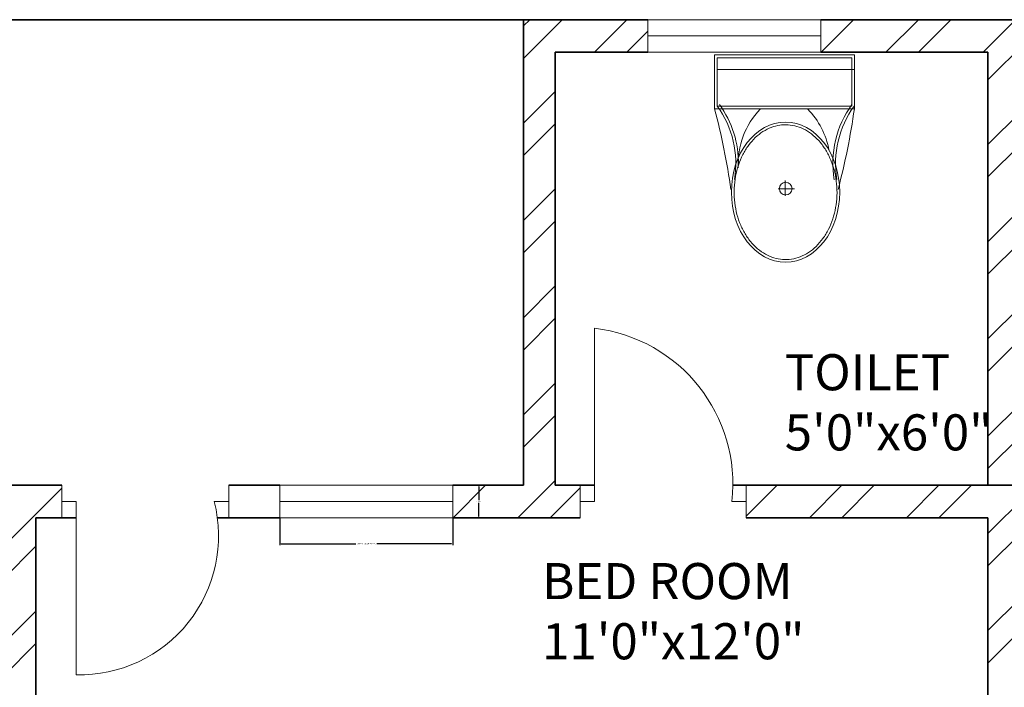
# Model space of a CAD drawing. Units: inches. Extents: x 2168 to 3056, y 1130 to 2629.
# Tile 31 of 42: x 2462 to 2598, y 2386 to 2478. Entities that reach past the tile are written whole.
import ezdxf

# ---------------------------------------------------------------- set-up
doc = ezdxf.new("R2010")
doc.units = ezdxf.units.IN
for name, color, linetype, lineweight in [('A-ANNO-DIMS', 2, 'Continuous', 18), ('A-AREA-IDEN', 7, 'Continuous', 18), ('A-DOOR', 21, 'Continuous', 18), ('A-FLOR-FIXT', 9, 'Continuous', 18), ('A-GLAZ', 201, 'Continuous', 18), ('A-WALL', 7, 'Continuous', 35)]:
    doc.layers.add(name, color=color, linetype=linetype, lineweight=lineweight)
doc.layers.add('A-WALL-PATT', color=143, linetype='Continuous', lineweight=13, true_color=0x7aafdf)
doc.styles.get("Standard").update_dxf_attribs({"font": 'arial.ttf'})
doc.dimstyles.get("Standard").update_dxf_attribs({"dimtxt": 0.18, "dimasz": 0.18, "dimexe": 0.18, "dimexo": 0.0625, "dimgap": 0.09, "dimtad": 0, "dimtih": 1, "dimtoh": 1, "dimdec": 4, "dimzin": 0, "dimdsep": 46, "dimtxsty": 'Standard', "dimcen": 0.09, "dimadec": 0, "dimazin": 0, "dimtfac": 1, "dimtdec": 4, "dimtofl": 0, "dimtmove": 0, "dimatfit": 3, "dimfxl": 1, "dimtolj": 1, "dimtzin": 0, "dimarcsym": 0})

# ---------------------------------------------------------------- blocks, each defined once
blk = doc.blocks.new('A$C31115884')
for p, q in [((257.5, 466.4), (257.5, 523.2)), ((283.1, 497.7), (223.4, 497.7)), ((0, 200), (0, 0)), ((520, 200), (0, 200)), ((10, 190), (10, 10)), ((510, 190), (10, 190)), ((510, 10), (510, 190)), ((520, 0), (520, 200)), ((510, 54.5), (0, 54.5)), ((10, 10), (510, 10)), ((0, 0), (520, 0))]:
    blk.add_line(p, q)
blk.add_circle((255.6, 496.4), 23.6)
for centre, radius, start, end in [((2777.7, -204.6), 2807, 165.4549, 171.7133), ((3237, 905), 2807, 188.2867, 194.5451), ((-294.5, 403.3), 364.7, 324.2091, 9.3499), ((-294.5, 403.3), 374.7, 324.2091, 9.3499), ((805.8, 403.3), 364.7, 170.6501, 215.7909), ((139.5, 406.2), 293.5, 315.8436, 2.6563), ((805.8, 403.3), 374.7, 179.2036, 215.7909), ((383.6, 406.2), 293.5, 190.2774, 224.1564)]:
    blk.add_arc(centre, radius, start, end)
blk.add_ellipse((256.2, 509.9), major_axis=(0, -260.7), ratio=0.772727)
blk.add_open_spline([(256.2, 259.2), (263.1, 259.2), (270, 259.7), (287.8, 262.3), (298.7, 265.1), (319.9, 273.1), (330.2, 278.4), (350.1, 291.1), (359.7, 298.7), (377.7, 315.9), (386.2, 325.5), (401.7, 346.6), (408.8, 358.1), (421.3, 382.5), (426.8, 395.5), (435.9, 422.4), (439.5, 436.4), (444.8, 465.1), (446.5, 479.7), (447.9, 509.2), (447.6, 524), (445, 553.3), (442.7, 567.8), (436.3, 596), (432.1, 609.7), (421.9, 636), (416, 648.6), (402.5, 672.1), (395, 683), (378.6, 703), (369.8, 712.1), (351.1, 728), (341.3, 734.8), (320.9, 746.2), (310.4, 750.7), (288.9, 757.3), (278, 759.4), (256, 761), (245, 760.6), (223.1, 757.2), (212.3, 754.3), (191.1, 746.1), (180.8, 740.7), (160.9, 727.8), (151.4, 720.1), (133.5, 702.7), (125.1, 693), (109.6, 671.7), (102.6, 660.2), (90.2, 635.7), (84.9, 622.7), (76, 595.6), (72.4, 581.6), (67.2, 552.9), (65.6, 538.2), (64.4, 508.8), (64.8, 494), (67.5, 464.7), (69.9, 450.2), (76.6, 422), (80.8, 408.3), (91.1, 382.2), (97.2, 369.7), (110.8, 346.3), (118.4, 335.4), (134.8, 315.6), (143.7, 306.7), (162.4, 290.9), (172.3, 284.2), (192.8, 273), (203.3, 268.6), (224.8, 262.2), (235.8, 260.2), (249.9, 259.3), (253, 259.2), (256.2, 259.2)], degree=3, knots=[0, 0, 0, 0, 0.110105, 0.110105, 0.285049, 0.285049, 0.459994, 0.459994, 0.634938, 0.634938, 0.809882, 0.809882, 0.984827, 0.984827, 1.159771, 1.159771, 1.334715, 1.334715, 1.50966, 1.50966, 1.684604, 1.684604, 1.859549, 1.859549, 2.034493, 2.034493, 2.209437, 2.209437, 2.384382, 2.384382, 2.559326, 2.559326, 2.73427, 2.73427, 2.909215, 2.909215, 3.084159, 3.084159, 3.259103, 3.259103, 3.434048, 3.434048, 3.608992, 3.608992, 3.783936, 3.783936, 3.958881, 3.958881, 4.133825, 4.133825, 4.30877, 4.30877, 4.483714, 4.483714, 4.658658, 4.658658, 4.833603, 4.833603, 5.008547, 5.008547, 5.183491, 5.183491, 5.358436, 5.358436, 5.53338, 5.53338, 5.708324, 5.708324, 5.883269, 5.883269, 6.058213, 6.058213, 6.233158, 6.233158, 6.283185, 6.283185, 6.283185, 6.283185])
blk = doc.blocks.new('WIN-24-OPPOSED-JAMBS')
for p, q in [((0, 4.5), (0, 0)), ((0, 4.5), (24, 4.5)), ((24, 2.25), (24, 4.5)), ((24, 4.5), (24, 0)), ((0, 0), (0, 2.25)), ((0, 2.25), (24, 2.25)), ((0, 0), (24, 0))]:
    blk.add_line(p, q)
blk = doc.blocks.new('WIN-24')
for p, q in [((0, 0), (0, 4.5)), ((0, 4.5), (0, 2.25)), ((0, 4.5), (24, 4.5)), ((24, 2.25), (24, 4.5)), ((24, 4.5), (24, 0)), ((0, 2.25), (24, 2.25)), ((24, 0), (0, 0))]:
    blk.add_line(p, q)
blk = doc.blocks.new('*D30')
at = {"layer": 'A-ANNO-DIMS', "color": 0, "lineweight": -2, "transparency": 16777216}
for p, q in [((2497.6, 2409.33), (2497.6, 2405.61)), ((2521.6, 2409.33), (2521.6, 2405.61)), ((2497.78, 2405.79), (2508.15, 2405.79)), ((2521.42, 2405.79), (2511.05, 2405.79))]:
    blk.add_line(p, q, dxfattribs=at)
at = {"layer": 'A-ANNO-DIMS', "color": 0, "transparency": 16777216}
for points in [[(2497.78, 2405.82), (2497.78, 2405.76), (2497.6, 2405.79)], [(2521.42, 2405.82), (2521.42, 2405.76), (2521.6, 2405.79)]]:
    blk.add_solid(points, dxfattribs=at)
at = {"layer": 'Defpoints', "color": 0, "transparency": 16777216}
for p in [(2497.6, 2409.39), (2521.6, 2409.39), (2521.6, 2405.79)]:
    blk.add_point(p, dxfattribs=at)
at = {"layer": 'A-ANNO-DIMS', "color": 0, "transparency": 16777216, "insert": (2509.6, 2405.79), "char_height": 0.18, "attachment_point": 5}
blk.add_mtext('\\A1;OPP. WINDOW 24 TYP.', dxfattribs=at)
blk = doc.blocks.new('*D31')
at = {"layer": 'A-ANNO-DIMS', "color": 0, "lineweight": -2, "transparency": 16777216}
for p, q in [((2521.66, 2413.89), (2525.38, 2413.89)), ((2525.2, 2413.71), (2525.2, 2411.82)), ((2525.2, 2409.57), (2525.2, 2411.46)), ((2521.66, 2409.39), (2525.38, 2409.39))]:
    blk.add_line(p, q, dxfattribs=at)
at = {"layer": 'A-ANNO-DIMS', "color": 0, "transparency": 16777216}
for points in [[(2525.17, 2413.71), (2525.23, 2413.71), (2525.2, 2413.89)], [(2525.17, 2409.57), (2525.23, 2409.57), (2525.2, 2409.39)]]:
    blk.add_solid(points, dxfattribs=at)
at = {"layer": 'Defpoints', "color": 0, "transparency": 16777216}
for p in [(2521.6, 2413.89), (2525.2, 2413.89), (2521.6, 2409.39)]:
    blk.add_point(p, dxfattribs=at)
at = {"layer": 'A-ANNO-DIMS', "color": 0, "transparency": 16777216, "insert": (2525.2, 2411.64), "char_height": 0.18, "attachment_point": 5}
blk.add_mtext('\\A1;5 TYP.', dxfattribs=at)

msp = doc.modelspace()

# ---------------------------------------------------------------- hatches: boundary and pattern name
at = {"layer": 'A-WALL-PATT'}
h = msp.add_hatch(dxfattribs=at)
h.set_pattern_fill('ANSI32', color=256)
h.paths.add_polyline_path([(2463.8, 2409.39), (2467.39, 2409.39), (2467.39, 2413.89), (2454.77, 2413.89), (2454.77, 2411.64), (2454.77, 2409.39), (2459.3, 2409.39), (2459.3, 2265.39), (2455.64, 2265.39), (2455.64, 2260.89), (2467.35, 2260.89), (2467.35, 2263.14), (2467.35, 2265.39), (2463.8, 2265.39)])
h.paths.add_polyline_path([(2431.6, 2413.89), (2409.65, 2413.89), (2409.65, 2409.39), (2431.6, 2409.39), (2431.6, 2411.64)])
h.paths.add_polyline_path([(2349.65, 2413.89), (2331.8, 2413.89), (2331.8, 2362.67), (2336.3, 2362.67), (2336.3, 2409.39), (2349.65, 2409.39), (2349.65, 2411.64)])
h.paths.add_polyline_path([(2634.15, 2411.64), (2634.15, 2413.89), (2562.29, 2413.89), (2562.29, 2409.39), (2595.8, 2409.39), (2595.8, 2280.31), (2595.83, 2280.31), (2595.83, 2265.39), (2499.91, 2265.39), (2499.91, 2260.89), (2550.8, 2260.89), (2550.8, 2117.31), (2555.3, 2117.31), (2555.3, 2168.08), (2571.93, 2168.08), (2571.93, 2176.89), (2559.8, 2176.89), (2559.8, 2256.39), (2640.8, 2256.39), (2640.8, 2176.89), (2626.43, 2176.89), (2626.43, 2168.08), (2645.3, 2168.08), (2645.3, 2116.64), (2649.8, 2116.64), (2649.8, 2260.89), (2691.25, 2260.89), (2691.25, 2263.14), (2691.25, 2265.39), (2670.65, 2265.39), (2670.65, 2265.36), (2600.3, 2265.36), (2600.3, 2280.26), (2600.3, 2409.39), (2634.15, 2409.39)])
h.paths.add_polyline_path([(2600.3, 2473.89), (2612.84, 2473.89), (2612.84, 2478.39), (2572.64, 2478.39), (2572.64, 2473.89), (2595.8, 2473.89), (2595.8, 2413.89), (2600.3, 2413.89)])
h.paths.add_polyline_path([(2535.8, 2473.89), (2548.64, 2473.89), (2548.64, 2478.39), (2531.4, 2478.39), (2531.4, 2413.89), (2521.6, 2413.89), (2521.6, 2409.39), (2539.24, 2409.39), (2539.24, 2411.64), (2539.24, 2413.89), (2535.8, 2413.89)])
h.paths.add_polyline_path([(2664.8, 2478.39), (2636.84, 2478.39), (2636.84, 2473.89), (2660.3, 2473.89), (2660.3, 2413.89), (2656.17, 2413.89), (2656.17, 2409.39), (2671.68, 2409.39), (2671.68, 2411.64), (2671.68, 2413.89), (2664.8, 2413.89)])
h.paths.add_polyline_path([(2705.94, 2413.89), (2695.68, 2413.89), (2695.68, 2409.39), (2705.94, 2409.39)])
h.paths.add_polyline_path([(2741.35, 2413.89), (2728.73, 2413.89), (2728.73, 2411.64), (2728.73, 2409.39), (2732.3, 2409.39), (2732.3, 2265.39), (2725.73, 2265.39), (2725.73, 2260.89), (2740.92, 2260.89), (2740.92, 2263.14), (2740.92, 2265.39), (2736.8, 2265.39), (2736.8, 2409.39), (2741.35, 2409.39)])
h.paths.add_polyline_path([(2785.65, 2413.89), (2764.55, 2413.89), (2764.49, 2409.39), (2785.65, 2409.39), (2785.65, 2411.64)])
h.paths.add_polyline_path([(2864.3, 2413.89), (2845.65, 2413.89), (2845.65, 2409.39), (2859.8, 2409.39), (2859.8, 2368.43), (2864.3, 2368.43)])
h.paths.add_polyline_path([(2864.3, 2308.43), (2862.05, 2308.43), (2859.8, 2308.43), (2859.8, 2265.39), (2774.48, 2265.39), (2774.48, 2263.14), (2774.48, 2260.89), (2781.8, 2260.89), (2781.8, 2226.65), (2786.3, 2226.65), (2786.3, 2260.89), (2859.8, 2260.89), (2859.8, 2241.35), (2864.3, 2241.35)])
h.paths.add_polyline_path([(2864.3, 2217.35), (2862.05, 2217.35), (2859.8, 2217.35), (2859.8, 2200.89), (2786.3, 2200.89), (2786.3, 2205.93), (2784.05, 2205.93), (2781.8, 2205.93), (2781.8, 2150.97), (2786.3, 2150.97), (2786.3, 2161.89), (2859.8, 2161.89), (2859.8, 2144.42), (2864.3, 2144.42)])
h.paths.add_polyline_path([(2859.8, 2196.39), (2859.8, 2166.39), (2786.3, 2166.39), (2786.3, 2196.39)], flags=16)
h.paths.add_polyline_path([(2864.3, 2108.42), (2862.05, 2108.42), (2859.8, 2108.42), (2859.8, 2080.89), (2786.3, 2080.89), (2786.3, 2111.99), (2781.8, 2111.99), (2781.8, 2080.89), (2649.8, 2080.89), (2649.8, 2086.04), (2647.55, 2086.04), (2645.3, 2086.04), (2645.3, 2071.74), (2649.8, 2071.74), (2649.8, 2076.39), (2781.8, 2076.39), (2781.8, 2041.79), (2786.3, 2041.79), (2786.3, 2076.39), (2859.8, 2076.39), (2859.8, 2058.58), (2864.3, 2058.58)])
h.paths.add_polyline_path([(2864.3, 2022.58), (2859.8, 2022.58), (2859.8, 1992.39), (2786.3, 1992.39), (2786.3, 1999.57), (2781.8, 1999.57), (2781.8, 1848.09), (2784.05, 1848.09), (2786.3, 1848.09), (2786.3, 1851.39), (2859.8, 1851.39), (2859.8, 1838.26), (2864.3, 1838.26)], flags=17)
h.paths.add_polyline_path([(2859.8, 1987.89), (2859.8, 1855.89), (2786.3, 1855.89), (2786.3, 1987.89)], flags=16)
h.paths.add_polyline_path([(2823.05, 1987.89), (2841.42, 1921.89), (2823.05, 1855.89)], flags=0)
h.paths.add_polyline_path([(2864.3, 1814.26), (2859.8, 1814.26), (2859.8, 1791.39), (2786.3, 1791.39), (2786.3, 1825.66), (2784.05, 1825.66), (2781.8, 1825.66), (2781.8, 1791.39), (2720.15, 1791.39), (2720.15, 1791.27), (2649.8, 1791.27), (2649.8, 1806.16), (2649.8, 2038.98), (2647.55, 2038.98), (2645.3, 2038.98), (2645.3, 1783.93), (2649.8, 1783.93), (2649.8, 1786.89), (2781.8, 1786.89), (2781.8, 1746.79), (2786.3, 1746.79), (2786.3, 1786.89), (2859.8, 1786.89), (2859.8, 1770.08), (2864.3, 1770.08)])
h.paths.add_polyline_path([(2864.3, 1734.08), (2862.05, 1734.08), (2859.8, 1734.08), (2859.8, 1705.89), (2786.3, 1705.89), (2786.3, 1714.17), (2781.8, 1714.17), (2781.8, 1660.53), (2786.3, 1660.53), (2786.3, 1666.89), (2859.8, 1666.89), (2859.8, 1648.34), (2864.3, 1648.34)])
h.paths.add_polyline_path([(2786.3, 1701.39), (2859.8, 1701.39), (2859.8, 1671.39), (2786.3, 1671.39)], flags=16)
h.paths.add_polyline_path([(2649.8, 1756.58), (2647.55, 1756.58), (2645.3, 1756.58), (2645.3, 1606.89), (2555.3, 1606.89), (2555.3, 1749.51), (2553.05, 1749.51), (2550.8, 1749.51), (2550.8, 1606.89), (2503.01, 1606.89), (2503.01, 1604.64), (2503.01, 1602.39), (2595.8, 1602.39), (2595.85, 1602.39), (2595.85, 1587.5), (2595.8, 1458.39), (2561.5, 1458.39), (2561.5, 1456.14), (2561.5, 1453.89), (2595.8, 1453.89), (2595.8, 1381.89), (2573.44, 1381.89), (2573.44, 1377.39), (2613.01, 1377.39), (2613.01, 1379.64), (2613.01, 1381.89), (2600.3, 1381.89), (2600.3, 1453.89), (2634.33, 1453.89), (2634.33, 1458.39), (2600.3, 1458.39), (2600.3, 1602.39), (2670.65, 1602.39), (2694.09, 1602.39), (2694.09, 1606.89), (2649.8, 1606.89)])
h.paths.add_polyline_path([(2736.8, 1602.39), (2741.56, 1602.39), (2741.56, 1606.89), (2726.2, 1606.89), (2726.2, 1604.64), (2726.2, 1602.39), (2732.3, 1602.39), (2732.3, 1458.39), (2727.9, 1458.39), (2727.9, 1453.89), (2740.82, 1453.89), (2740.82, 1456.14), (2740.82, 1458.39), (2736.8, 1458.39)])
h.paths.add_polyline_path([(2859.8, 1606.89), (2786.3, 1606.89), (2786.3, 1637.33), (2784.05, 1637.33), (2781.8, 1637.33), (2781.8, 1606.89), (2775.61, 1606.89), (2775.61, 1602.39), (2859.8, 1602.39)])
h.paths.add_polyline_path([(2864.3, 1624.34), (2862.05, 1624.34), (2859.8, 1624.34), (2859.8, 1570.39), (2864.3, 1570.39)])
h.paths.add_polyline_path([(2864.3, 1510.39), (2862.05, 1510.39), (2859.8, 1510.39), (2859.8, 1458.39), (2846.73, 1458.39), (2846.73, 1456.14), (2846.73, 1453.89), (2864.3, 1453.89)])
h.paths.add_polyline_path([(2786.73, 1458.39), (2765.44, 1458.39), (2765.44, 1453.89), (2786.73, 1453.89)])
h.paths.add_polyline_path([(2706, 1458.39), (2695.36, 1458.39), (2695.36, 1453.89), (2706, 1453.89), (2706, 1456.14)])
h.paths.add_polyline_path([(2671.36, 1456.14), (2671.36, 1458.39), (2655.99, 1458.39), (2655.99, 1456.14), (2655.99, 1453.89), (2660.3, 1453.89), (2660.3, 1381.89), (2637.01, 1381.89), (2637.01, 1377.39), (2664.8, 1377.39), (2664.8, 1453.89), (2671.36, 1453.89)], flags=17)
h.paths.add_polyline_path([(2539.83, 1458.39), (2520.24, 1458.39), (2520.24, 1453.89), (2531.3, 1453.89), (2531.3, 1377.39), (2546.45, 1377.39), (2546.45, 1379.64), (2546.45, 1381.89), (2535.8, 1381.89), (2535.8, 1453.89), (2539.83, 1453.89)], flags=17)
h.paths.add_polyline_path([(2496.24, 1458.39), (2489.13, 1458.39), (2489.13, 1453.89), (2496.24, 1453.89), (2496.24, 1456.14)])
h.paths.add_polyline_path([(2467.43, 1456.14), (2467.43, 1458.39), (2463.8, 1458.39), (2463.8, 1602.39), (2468.24, 1602.39), (2468.24, 1605.7), (2468.24, 1606.89), (2454.6, 1606.89), (2454.6, 1602.39), (2459.3, 1602.39), (2459.3, 1458.39), (2454.24, 1458.39), (2454.24, 1453.89), (2467.43, 1453.89)])
h.paths.add_polyline_path([(2431.6, 1456.14), (2431.6, 1458.39), (2411.39, 1458.39), (2411.39, 1453.89), (2431.6, 1453.89)])
h.paths.add_polyline_path([(2351.39, 1458.39), (2336.3, 1458.39), (2336.3, 1490.69), (2334.05, 1490.69), (2331.8, 1490.69), (2331.8, 1453.89), (2351.39, 1453.89), (2351.39, 1456.14)])
h.paths.add_polyline_path([(2336.3, 1629.7), (2331.8, 1629.7), (2331.8, 1552.32), (2336.3, 1552.32), (2336.3, 1602.39), (2406.65, 1602.39), (2423.47, 1602.39), (2423.47, 1606.89), (2418.8, 1606.89), (2418.8, 1643.68), (2416.55, 1643.68), (2414.3, 1643.68), (2414.3, 1606.89), (2336.3, 1606.89)])
h.paths.add_polyline_path([(2418.8, 1714.38), (2414.3, 1714.38), (2414.3, 1705.89), (2336.3, 1705.89), (2336.3, 1731.32), (2334.05, 1731.32), (2331.8, 1731.32), (2331.8, 1653.7), (2334.05, 1653.7), (2336.3, 1653.7), (2336.3, 1666.89), (2414.3, 1666.89), (2414.3, 1663.59), (2418.8, 1663.59)])
h.paths.add_polyline_path([(2336.3, 1701.39), (2414.3, 1701.39), (2414.3, 1671.39), (2336.3, 1671.39)], flags=16)
h.paths.add_polyline_path([(2555.3, 2040.06), (2550.8, 2040.06), (2550.8, 1791.39), (2550.56, 1791.2), (2480.2, 1791.2), (2418.8, 1791.39), (2418.8, 1825.45), (2416.55, 1825.45), (2414.3, 1825.45), (2414.3, 1791.39), (2336.3, 1791.39), (2336.3, 1806.41), (2331.8, 1806.41), (2331.8, 1767.32), (2336.3, 1767.32), (2336.3, 1786.89), (2414.3, 1786.89), (2414.3, 1745.46), (2418.8, 1745.46), (2418.8, 1786.89), (2550.8, 1786.89), (2550.8, 1783.01), (2555.3, 1783.01)])
h.paths.add_polyline_path([(2418.8, 1923.39), (2423.21, 1923.39), (2423.21, 1925.64), (2423.21, 1927.89), (2418.8, 1927.89), (2418.8, 2000.05), (2414.3, 2000.05), (2414.3, 1992.39), (2336.3, 1992.39), (2336.3, 1987.89), (2414.3, 1987.89), (2414.3, 1855.89), (2336.3, 1855.89), (2336.3, 1851.39), (2414.3, 1851.39), (2414.3, 1846.76), (2418.8, 1846.76)], flags=17)
h.paths.add_polyline_path([(2336.3, 2019.29), (2334.05, 2019.29), (2331.8, 2019.29), (2331.8, 1830.41), (2336.3, 1830.41)], flags=17)
h.paths.add_polyline_path([(2550.8, 1927.89), (2453.54, 1927.89), (2453.54, 1925.64), (2453.54, 1923.39), (2550.8, 1923.39)], flags=17)
h.paths.add_polyline_path([(2744.99, 1927.89), (2649.8, 1927.89), (2649.8, 1923.39), (2744.99, 1923.39), (2744.99, 1925.64)], flags=17)
h.paths.add_polyline_path([(2555.3, 2086.46), (2553.05, 2086.46), (2550.8, 2086.46), (2550.8, 2080.89), (2418.8, 2080.89), (2336.3, 2080.89), (2336.3, 2115.4), (2334.05, 2115.4), (2331.8, 2115.4), (2331.8, 2055.29), (2336.3, 2055.29), (2336.3, 2076.39), (2550.8, 2076.39), (2550.8, 2071.54), (2555.3, 2071.54)])
h.paths.add_polyline_path([(2418.8, 2121.39), (2414.3, 2121.39), (2414.3, 2080.89), (2418.8, 2080.89)])
h.paths.add_polyline_path([(2418.8, 2076.39), (2414.3, 2076.39), (2414.3, 2035.12), (2418.8, 2035.12)])
h.paths.add_polyline_path([(2422.87, 2263.14), (2422.87, 2265.39), (2406.65, 2265.39), (2406.65, 2265.36), (2336.3, 2265.36), (2336.3, 2280.25), (2336.3, 2302.67), (2334.05, 2302.67), (2331.8, 2302.67), (2331.8, 2246.85), (2336.3, 2246.85), (2336.3, 2260.89), (2414.3, 2260.89), (2414.3, 2224), (2418.8, 2224), (2418.8, 2260.89), (2422.87, 2260.89)])
h.paths.add_polyline_path([(2418.8, 2204.78), (2416.55, 2204.78), (2414.3, 2204.78), (2414.3, 2200.89), (2336.3, 2200.89), (2336.3, 2220.85), (2331.8, 2220.85), (2331.8, 2151.4), (2336.3, 2151.4), (2336.3, 2161.89), (2414.3, 2161.89), (2414.3, 2153.73), (2418.8, 2153.73)])
h.paths.add_polyline_path([(2414.3, 2196.39), (2414.3, 2166.39), (2336.3, 2166.39), (2336.3, 2196.39)], flags=16)
h.paths.add_polyline_path([(2375.3, 2181.39), (2336.3, 2166.39), (2336.3, 2196.39)], flags=0)
h.paths.add_polyline_path([(2809.6, 2172.34), (2838.8, 2172.34), (2838.8, 2191), (2809.6, 2191)], flags=8)
h.paths.add_polyline_path([(2849.75, 1919.59), (2849.75, 1952.67), (2831.09, 1952.67), (2831.09, 1919.59)], flags=8)
h.paths.add_polyline_path([(2808.87, 1901.97), (2808.87, 1937.85), (2790.15, 1937.85), (2790.15, 1901.97)], flags=8)
h.paths.add_polyline_path([(2806.28, 1671.9), (2835.49, 1671.9), (2835.49, 1690.55), (2806.28, 1690.55)], flags=8)
h.paths.add_polyline_path([(2353.19, 1676.55), (2382.39, 1676.55), (2382.39, 1695.21), (2353.19, 1695.21)], flags=8)
h.paths.add_polyline_path([(2360.08, 1832.31), (2389.24, 1832.31), (2389.24, 1850.97), (2360.08, 1850.97)], flags=25)
h.paths.add_polyline_path([(2354.82, 2167.82), (2384.03, 2167.82), (2384.03, 2186.48), (2354.82, 2186.48)], flags=8)

# ---------------------------------------------------------------- linework, layer by layer
at = {"layer": 'A-DOOR'}
for p, q in [((2541.24, 2411.64), (2541.24, 2435.64)), ((2467.39, 2409.39), (2467.39, 2413.89)), ((2467.39, 2413.89), (2467.39, 2411.64)), ((2490.52, 2413.89), (2490.52, 2409.39)), ((2539.24, 2413.89), (2539.24, 2409.39)), ((2562.29, 2413.89), (2562.29, 2409.39)), ((2467.39, 2411.64), (2467.39, 2411.64)), ((2467.39, 2411.64), (2469.39, 2411.64)), ((2469.39, 2411.64), (2469.39, 2387.64)), ((2490.52, 2411.64), (2488.52, 2411.64)), ((2490.52, 2409.39), (2490.52, 2411.64)), ((2539.24, 2409.39), (2539.24, 2411.64)), ((2539.24, 2411.64), (2541.24, 2411.64)), ((2562.29, 2411.64), (2560.29, 2411.64)), ((2562.29, 2409.39), (2562.29, 2411.64))]:
    msp.add_line(p, q, dxfattribs=at)
for centre, radius, start, end in [((2538.68, 2414.04), 21.75, 353.649, 83.2438), ((2469.89, 2406.86), 19.23, 268.4939, 14.3776)]:
    msp.add_arc(centre, radius, start, end, dxfattribs=at)
at = {"layer": 'A-WALL'}
for p, q in [((2331.8, 2478.39), (2548.64, 2478.39)), ((2531.4, 2478.39), (2531.4, 2413.89)), ((2572.64, 2478.39), (2612.84, 2478.39)), ((2535.8, 2473.89), (2548.64, 2473.89)), ((2535.8, 2413.89), (2535.8, 2473.89)), ((2572.64, 2473.89), (2595.8, 2473.89)), ((2595.8, 2473.89), (2595.8, 2413.89)), ((2454.77, 2413.89), (2467.39, 2413.89)), ((2490.52, 2413.89), (2497.6, 2413.89)), ((2521.6, 2413.89), (2531.4, 2413.89)), ((2535.8, 2413.89), (2541.24, 2413.89)), ((2541.24, 2413.89), (2535.8, 2413.89)), ((2595.8, 2413.89), (2560.43, 2413.89)), ((2560.43, 2413.89), (2635.64, 2413.89)), ((2463.8, 2409.39), (2463.8, 2265.39)), ((2463.8, 2409.39), (2469.39, 2409.39)), ((2488.96, 2409.39), (2497.6, 2409.39)), ((2521.6, 2409.39), (2539.24, 2409.39)), ((2562.29, 2409.39), (2595.8, 2409.39)), ((2595.8, 2409.39), (2595.8, 2265.39))]:
    msp.add_line(p, q, dxfattribs=at)

# ---------------------------------------------------------------- block references
at = {"layer": 'A-FLOR-FIXT', "xscale": 0.0372717239612423, "yscale": 0.0372717239612423, "zscale": 0.0372717239612423, "rotation": 180}
msp.add_blockref('A$C31115884', (2577.28, 2473.5), dxfattribs=at)
at = {"layer": 'A-GLAZ'}
for name, p in [('WIN-24', (2548.64, 2473.89)), ('WIN-24-OPPOSED-JAMBS', (2497.6, 2409.39))]:
    msp.add_blockref(name, p, dxfattribs=at)

# ---------------------------------------------------------------- texts
at = {"layer": 'A-AREA-IDEN', "char_height": 5, "attachment_point": 1}
for s, width, insert in [('TOILET\\P5\'0"x6\'0"', 116.5731, (2567.62, 2432.05)), ('BED ROOM\\P11\'0"x12\'0"', 197.9433, (2533.98, 2403.11))]:
    msp.add_mtext_dynamic_manual_height_columns(s, width=width, gutter_width=12.5, heights=[0], dxfattribs=dict(at, insert=insert))

# ---------------------------------------------------------------- dimensions: what is measured, and where the dimension line sits
at = {"layer": 'A-ANNO-DIMS'}
dim = msp.add_linear_dim(base=(2525.19989217, 2413.88887054), p1=(2521.59989217, 2409.38887054), p2=(2521.59989217, 2413.88887054), angle=90, text='<> TYP.', dimstyle='Standard', override={"dimdec": 0, "dimlfac": 1, "dimrnd": 0, "dimzin": 0, "dimdsep": 46, "dimlunit": 2}, dxfattribs=at)
dim.commit()
dim.dimension.update_dxf_attribs({"geometry": '*D31', "text_midpoint": (2525.19989217, 2411.63887054)})
dim = msp.add_linear_dim(base=(2521.6, 2405.79), p1=(2497.6, 2409.39), p2=(2521.6, 2409.39), text='OPP. WINDOW <> TYP.', dimstyle='Standard', override={"dimdec": 0, "dimlfac": 1, "dimrnd": 0, "dimzin": 0, "dimdsep": 46, "dimlunit": 2}, dxfattribs=at)
dim.commit()
dim.dimension.update_dxf_attribs({"geometry": '*D30', "text_midpoint": (2509.6, 2405.79)})

doc.saveas('drawing.dxf')
